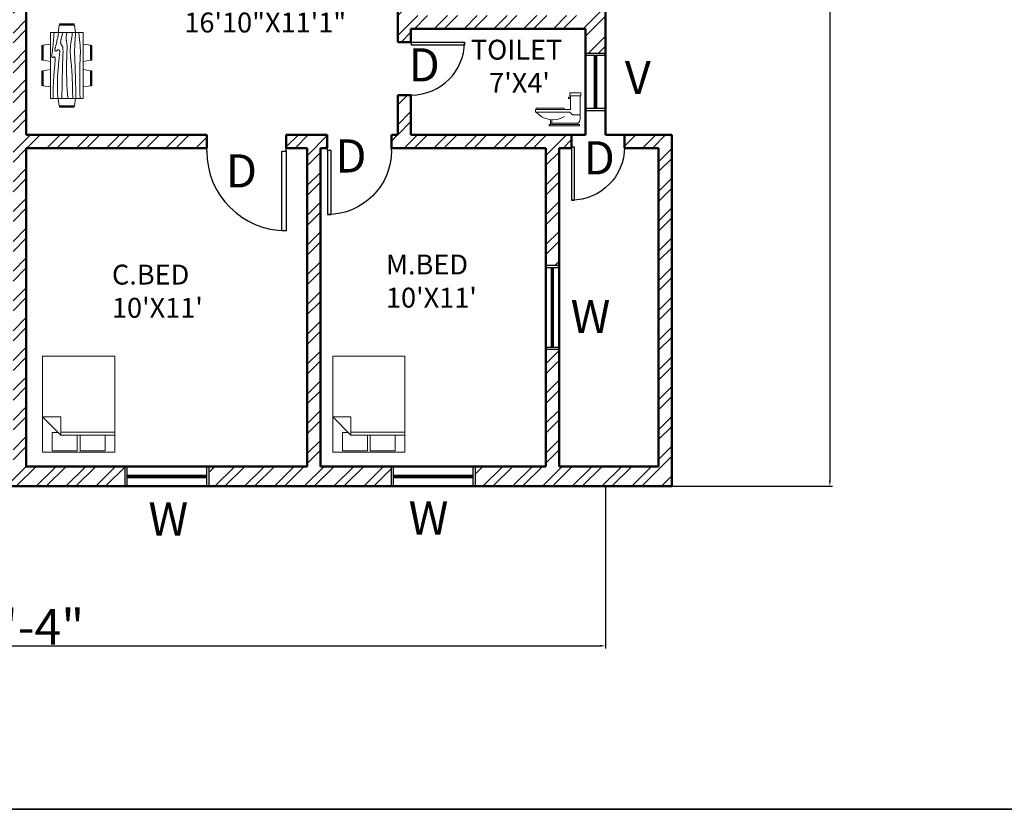
# Model space of a CAD drawing. Units: inches. Extents: x -31842 to -29388, y 18869 to 19743.
# Tile 7 of 12: x -30617 to -30172, y 18869 to 19226. Entities that reach past the tile are written whole.
import ezdxf

# ---------------------------------------------------------------- set-up
doc = ezdxf.new("R2010")
doc.units = ezdxf.units.IN
for name, color, linetype, lineweight in [('A-ANNO-DIMS', 2, 'Continuous', 18), ('A-ANNO-SYMB', 2, 'Continuous', 18), ('A-ANNO-TTLB', 7, 'Continuous', 35), ('A-AREA-IDEN', 3, 'Continuous', 18), ('A-DOOR', 3, 'Continuous', 25), ('A-FLOR-FIXT', 8, 'Continuous', 18), ('A-FURN', 8, 'Continuous', 18), ('A-GLAZ', 4, 'Continuous', 25), ('A-WALL', 7, 'Continuous', 50), ('A-WALL-PATT', 8, 'Continuous', 13)]:
    doc.layers.add(name, color=color, linetype=linetype, lineweight=lineweight)
doc.styles.get("Standard").update_dxf_attribs({"font": 'arial.ttf'})
doc.dimstyles.new('ISO-25', dxfattribs={"dimtxt": 2.5, "dimasz": 2.5, "dimexe": 1.25, "dimexo": 0.625, "dimtad": 1, "dimdec": 0, "dimlunit": 3, "dimtxsty": 'Standard', "dimcen": 2.5, "dimadec": 0, "dimazin": 0, "dimtfac": 1, "dimtdec": 0, "dimtmove": 0, "dimatfit": 3, "dimfxl": 1, "dimarcsym": 0})

# ---------------------------------------------------------------- blocks, each defined once
blk = doc.blocks.new('*U8')
for p, q in [((0, 0), (0, -100)), ((750, 0), (750, -100))]:
    blk.add_line(p, q)
blk.add_lwpolyline([(0, 0), (0, 750), (43.75, 750), (43.75, 0)], close=True)
blk.add_arc((0, 0), 750, 0, 90)
blk = doc.blocks.new('Bed - Queen')
for p, q in [((0, -80.00003), (0, 0)), ((0, 0), (59.99999, 0)), ((59.99999, 0), (59.99999, -80.00003)), ((7.99999, -1.2), (28.79998, -1.2)), ((7.99999, -14.4), (7.99999, -1.2)), ((28.79998, -1.2), (28.79998, -14.4)), ((31.19999, -1.2), (51.99999, -1.2)), ((31.19999, -14.4), (31.19999, -1.2)), ((51.99999, -1.2), (51.99999, -16.4)), ((0, -14.4), (44.8, -14.4)), ((59.99999, -29.6), (44.8, -14.4)), ((44.8, -14.4), (44.8, -29.6)), ((44.8, -16.8), (0, -16.8)), ((51.99999, -16.4), (46.79936, -16.4)), ((44.8, -29.6), (59.99999, -29.6)), ((59.99999, -80.00003), (0, -80.00003))]:
    blk.add_line(p, q)
blk = doc.blocks.new('Toilet - side')
for p, q in [((0.5, 5), (0.5, 22)), ((7.5, 22), (7.5, 12)), ((7.5, 21), (9, 21)), ((9, 20), (7.5, 20)), ((9, 21), (9, 20)), ((6, 8), (0.5, 8)), ((8, 10), (6, 8)), ((7.5, 12), (33, 12)), ((33, 10), (8, 10)), ((32.5, 13), (12, 13)), ((12, 13), (12, 12)), ((32.5, 12), (32.5, 13)), ((33, 12), (33, 10)), ((22, 2), (2, 2)), ((2, 2), (2, 1)), ((21, 4.5), (21, 2)), ((22, 2), (22, 4.54)), ((22, 1), (22, 2))]:
    blk.add_line(p, q)
for points in [[(0, 22), (0, 24), (8, 24), (8, 22)], [(1, 0), (1, 1), (23, 1), (23, 0)]]:
    blk.add_lwpolyline(points, close=True)
for centre, radius, start, end in [((20.3, 20.7), 16.23, 238.18715, 318.77023), ((3.75, 4.75), 3.26, 175.6013, 237.5288)]:
    blk.add_arc(centre, radius, start, end)
blk = doc.blocks.new('Dining Set - 36 x 72 in.')
for p, q in [((-22.2343, 26.00059), (-23.4847, 17.99762)), ((-22.2304, 26), (-5.7608, 26)), ((-22, 27.5), (-22.1562, 26.50042)), ((-5.8416, 26.5), (-22.1534, 26.5)), ((-22, 27.5), (-6, 27.5)), ((-5.8437, 26.49966), (-6, 27.5)), ((-4.5152, 17.99762), (-5.7655, 25.99926)), ((5.7657, 26.00059), (4.5153, 17.99762)), ((5.7696, 26), (22.2392, 26)), ((6, 27.5), (5.8438, 26.50042)), ((22.1584, 26.5), (5.8466, 26.5)), ((6, 27.5), (22, 27.5)), ((22.1563, 26.49966), (22, 27.5)), ((23.4848, 17.99762), (22.2345, 25.99926)), ((36, 18), (-36, 18)), ((-36, 18), (-36, -18)), ((36, -18), (36, 18)), ((-45.5, 8), (-44.5004, 8.15617)), ((-45.5, 8), (-45.5, -8)), ((-44.5, -8.15843), (-44.5, 8.15338)), ((-44.0006, 8.23428), (-35.9976, 9.48474)), ((-44, 8.23041), (-44, -8.23915)), ((44.0006, 8.23428), (35.9976, 9.48474)), ((44, 8.23041), (44, -8.23915)), ((44.5, -8.15843), (44.5, 8.15338)), ((45.5, 8), (44.5005, 8.15617)), ((45.5, 8), (45.5, -8)), ((-44.4997, -8.15631), (-45.5, -8)), ((-35.9976, -9.48476), (-43.9993, -8.2345)), ((35.9976, -9.48476), (43.9993, -8.2345)), ((44.4997, -8.15631), (45.5, -8)), ((-36, -18), (36, -18)), ((-22.2343, -26.0006), (-23.4847, -17.99762)), ((-4.5152, -17.99762), (-5.7655, -25.99928)), ((5.7657, -26.0006), (4.5153, -17.99762)), ((23.4848, -17.99762), (22.2345, -25.99928)), ((-22.2304, -26), (-5.7608, -26)), ((-22, -27.5), (-22.1562, -26.50044)), ((-5.8416, -26.5), (-22.1534, -26.5)), ((-22, -27.5), (-6, -27.5)), ((-5.8437, -26.49967), (-6, -27.5)), ((5.7696, -26), (22.2392, -26)), ((6, -27.5), (5.8438, -26.50044)), ((22.1584, -26.5), (5.8466, -26.5)), ((6, -27.5), (22, -27.5)), ((22.1563, -26.49967), (22, -27.5))]:
    blk.add_line(p, q)
for points in [[(-36, 15), (-31.1772, 14.97754), (-26.8079, 14.91406), (-22.8538, 14.81543), (-19.276, 14.6875), (-16.0362, 14.53613), (-13.0957, 14.36718), (-10.4159, 14.18652), (-7.9583, 14), (-5.6904, 13.81315), (-3.6035, 13.63021), (-1.6954, 13.45508), (0.0365, 13.29166), (1.5945, 13.14388), (2.9811, 13.01562), (4.1988, 12.9108), (5.25, 12.83333), (6.1393, 12.78613), (6.8802, 12.76823), (7.4883, 12.77767), (7.9792, 12.8125), (8.3685, 12.87077), (8.6719, 12.95052), (8.9049, 13.0498), (9.0833, 13.16666), (9.2205, 13.29899), (9.3216, 13.44401), (9.3895, 13.59879), (9.4271, 13.76041), (9.4373, 13.92594), (9.4232, 14.09245), (9.3875, 14.257), (9.3333, 14.41666), (9.2638, 14.56917), (9.1836, 14.71484), (9.0975, 14.85465), (9.0104, 14.98958), (8.9272, 15.1206), (8.8529, 15.2487), (8.7922, 15.37483), (8.75, 15.5), (8.7305, 15.62467), (8.7344, 15.74739), (8.7617, 15.86621), (8.8125, 15.97916), (8.8867, 16.08431), (8.9844, 16.17968), (9.1055, 16.26334), (9.25, 16.33333), (9.4189, 16.38802), (9.6172, 16.42708), (9.8506, 16.45052), (10.125, 16.45833), (10.4463, 16.45052), (10.8203, 16.42708), (11.2529, 16.38802), (11.75, 16.33333), (12.3184, 16.26318), (12.9694, 16.17838), (13.7151, 16.07991), (14.5677, 15.96875), (15.5395, 15.84586), (16.6426, 15.71224), (17.8893, 15.56884), (19.2917, 15.41666), (20.859, 15.25667), (22.5879, 15.08984), (24.4721, 14.91715), (26.5052, 14.73958), (28.6809, 14.5581), (30.9929, 14.3737), (33.4347, 14.18733), (36, 14)], [(-36, 10), (-28.9766, 10.14274), (-23.1725, 10.20442), (-18.4241, 10.19775), (-14.5677, 10.13541), (-11.4399, 10.03011), (-8.877, 9.89453), (-6.7154, 9.74137), (-4.7917, 9.58333), (-2.9698, 9.43082), (-1.2246, 9.28515), (0.4415, 9.14534), (2.026, 9.01041), (3.5266, 8.87939), (4.9408, 8.7513), (6.266, 8.62516), (7.5, 8.5), (8.6411, 8.37549), (9.6914, 8.2539), (10.6538, 8.13818), (11.5312, 8.03125), (12.3267, 7.93603), (13.043, 7.85547), (13.6831, 7.79248), (14.25, 7.75), (14.7471, 7.7303), (15.1797, 7.73307), (15.5537, 7.75732), (15.875, 7.80208), (16.1494, 7.86637), (16.3828, 7.94922), (16.5811, 8.04964), (16.75, 8.16666), (16.8944, 8.29915), (17.0143, 8.44531), (17.1089, 8.60319), (17.1771, 8.77083), (17.218, 8.94629), (17.2305, 9.1276), (17.2137, 9.31282), (17.1667, 9.5), (17.0895, 9.6875), (16.987, 9.875), (16.8649, 10.0625), (16.7292, 10.25), (16.5856, 10.4375), (16.4401, 10.625), (16.2985, 10.8125), (16.1667, 11), (16.05, 11.18733), (15.9518, 11.3737), (15.8752, 11.5581), (15.8229, 11.73958), (15.798, 11.91715), (15.8034, 12.08984), (15.842, 12.25667), (15.9167, 12.41666), (16.0295, 12.56836), (16.1784, 12.70833), (16.3605, 12.83268), (16.5729, 12.9375), (16.8127, 13.01888), (17.0768, 13.07291), (17.3625, 13.0957), (17.6667, 13.08333), (17.9894, 13.03312), (18.3418, 12.94726), (18.7382, 12.82918), (19.1927, 12.68229), (19.7195, 12.51001), (20.3327, 12.31575), (21.0465, 12.10294), (21.875, 11.875), (22.8357, 11.63354), (23.959, 11.37304), (25.2786, 11.08618), (26.8282, 10.76562), (28.6414, 10.40405), (30.752, 9.99414), (33.1936, 9.52856), (36, 9)], [(-36, 5.5), (-30.7157, 5.3348), (-26.069, 5.20963), (-21.9946, 5.11767), (-18.4271, 5.05208), (-15.3009, 5.00602), (-12.5508, 4.97265), (-10.1112, 4.94515), (-7.9167, 4.91666), (-5.909, 4.88167), (-4.0586, 4.83984), (-2.3429, 4.79215), (-0.7396, 4.73958), (0.7739, 4.6831), (2.22, 4.6237), (3.6213, 4.56233), (5, 4.5), (6.373, 4.43782), (7.7344, 4.3776), (9.0723, 4.32129), (10.375, 4.27083), (11.6309, 4.22819), (12.8281, 4.19531), (13.9551, 4.17415), (15, 4.16666), (15.954, 4.17448), (16.819, 4.19791), (17.6001, 4.23698), (18.3021, 4.29166), (18.9299, 4.36198), (19.4883, 4.44791), (19.9823, 4.54948), (20.4167, 4.66666), (20.7969, 4.79899), (21.1302, 4.94401), (21.4245, 5.09879), (21.6875, 5.26041), (21.9271, 5.42594), (22.1511, 5.59245), (22.3672, 5.757), (22.5834, 5.91666), (22.8065, 6.06868), (23.0404, 6.21093), (23.2879, 6.34147), (23.5521, 6.45833), (23.8358, 6.55957), (24.142, 6.64323), (24.4735, 6.70735), (24.8334, 6.75), (25.2235, 6.76969), (25.642, 6.76692), (26.0858, 6.74267), (26.5521, 6.69791), (27.0379, 6.63362), (27.5404, 6.55078), (28.0565, 6.45036), (28.5834, 6.33333), (29.1242, 6.19987), (29.7071, 6.04687), (30.3661, 5.87044), (31.1354, 5.66666), (32.0493, 5.43164), (33.142, 5.16146), (34.4475, 4.85221), (36, 4.5)], [(-36, -1), (-30.7915, -0.6591), (-26.0195, -0.38216), (-21.6519, -0.16284), (-17.6563, 0.00521), (-14.0005, 0.12833), (-10.6523, 0.21289), (-7.5796, 0.26522), (-4.75, 0.29166), (-2.134, 0.29793), (0.2878, 0.28711), (2.5317, 0.26163), (4.6146, 0.22396), (6.5529, 0.17651), (8.3633, 0.12174), (10.0623, 0.06209), (11.6667, 0), (13.1899, -0.06201), (14.6341, -0.1211), (15.9982, -0.17432), (17.2813, -0.21875), (18.4823, -0.25147), (19.6003, -0.26953), (20.6343, -0.27002), (21.5834, -0.25), (22.4481, -0.20768), (23.2357, -0.14584), (23.9549, -0.06836), (24.6146, 0.02083), (25.2235, 0.11784), (25.7904, 0.21875), (26.3241, 0.31966), (26.8334, 0.41666), (27.3265, 0.50618), (27.8099, 0.58593), (28.2894, 0.65397), (28.7709, 0.70833), (29.2601, 0.74707), (29.763, 0.76823), (30.2855, 0.76985), (30.8334, 0.75), (31.4088, 0.70784), (31.9994, 0.64713), (32.589, 0.57275), (33.1615, 0.48958), (33.7008, 0.4025), (34.1908, 0.3164), (34.6153, 0.23616), (34.9584, 0.16666), (35.2099, 0.11165), (35.3848, 0.07031), (35.504, 0.04069), (35.5886, 0.02083), (35.6594, 0.00879), (35.7377, 0.0026), (35.8442, 0.00032), (36, 0)], [(-36, -6.5), (-27.1843, -6.31267), (-20.084, -6.1263), (-14.469, -5.9419), (-10.1094, -5.76042), (-6.7752, -5.58285), (-4.2363, -5.41016), (-2.2629, -5.24333), (-0.625, -5.08334), (0.8708, -4.93099), (2.2715, -4.78646), (3.5872, -4.64974), (4.8281, -4.52084), (6.0046, -4.39974), (7.127, -4.28646), (8.2053, -4.18099), (9.25, -4.08334), (10.2705, -3.99382), (11.2734, -3.91407), (12.2647, -3.84603), (13.25, -3.79167), (14.2354, -3.75293), (15.2266, -3.73177), (16.2295, -3.73015), (17.25, -3.75), (18.2912, -3.79248), (19.3451, -3.85547), (20.4009, -3.93604), (21.4479, -4.03125), (22.4754, -4.13819), (23.4727, -4.25391), (24.4289, -4.37549), (25.3334, -4.5), (26.1785, -4.62492), (26.9694, -4.74935), (27.7145, -4.87281), (28.4219, -4.99479), (29.1, -5.11483), (29.7572, -5.23242), (30.4016, -5.34709), (31.0417, -5.45834), (31.6837, -5.56437), (32.3262, -5.65821), (32.9658, -5.73153), (33.599, -5.77604), (34.2224, -5.78345), (34.8327, -5.74545), (35.4264, -5.65373), (36, -5.5)], [(-36, -10), (-26.4022, -9.81299), (-18.4675, -9.62891), (-11.9839, -9.45069), (-6.7396, -9.28125), (-2.5226, -9.12354), (0.8789, -8.98047), (3.6769, -8.85498), (6.0833, -8.75), (8.2767, -8.66765), (10.3021, -8.60677), (12.1712, -8.56543), (13.8958, -8.54167), (15.4876, -8.53353), (16.9583, -8.53907), (18.3197, -8.55632), (19.5834, -8.58334), (20.7616, -8.61841), (21.8685, -8.66081), (22.9188, -8.71004), (23.9271, -8.76563), (24.9081, -8.82707), (25.8763, -8.89388), (26.8465, -8.96558), (27.8334, -9.04167), (28.8474, -9.12118), (29.8828, -9.20117), (30.93, -9.27824), (31.9792, -9.34896), (33.0205, -9.40991), (34.0443, -9.45768), (35.0407, -9.48885), (36, -9.5)], [(-36, -14.5), (-30.0881, -14.33513), (-25.0332, -14.21224), (-20.7312, -14.12647), (-17.0781, -14.07292), (-13.97, -14.04671), (-11.3027, -14.04297), (-8.9724, -14.05681), (-6.875, -14.08334), (-4.9224, -14.11833), (-3.0905, -14.16016), (-1.3709, -14.20785), (0.2448, -14.26042), (1.7647, -14.3169), (3.1973, -14.3763), (4.5507, -14.43767), (5.8333, -14.5), (7.0554, -14.5621), (8.235, -14.62175), (9.3922, -14.67652), (10.5469, -14.72396), (11.7192, -14.76164), (12.929, -14.78711), (14.1965, -14.79794), (15.5417, -14.79167), (16.9933, -14.76424), (18.6152, -14.70508), (20.4804, -14.60197), (22.6615, -14.44271), (25.2312, -14.21509), (28.2624, -13.9069), (31.8277, -13.50594), (36, -13)]]:
    blk.add_lwpolyline(points)
blk = doc.blocks.new('*D203')
at = {"layer": 'A-ANNO-DIMS', "color": 0, "lineweight": -2, "transparency": 16777216}
for p, q in [((-30351.77, 19614.99), (-30249.67, 19614.99)), ((-30250.92, 19612.49), (-30250.92, 19017.46)), ((-30351.77, 19014.96), (-30249.67, 19014.96))]:
    blk.add_line(p, q, dxfattribs=at)
at = {"layer": 'A-ANNO-DIMS', "color": 0, "transparency": 16777216}
for points in [[(-30251.34, 19612.49), (-30250.5, 19612.49), (-30250.92, 19614.99)], [(-30251.34, 19017.46), (-30250.5, 19017.46), (-30250.92, 19014.96)]]:
    blk.add_solid(points, dxfattribs=at)
at = {"layer": 'Defpoints', "color": 0, "transparency": 16777216}
for p in [(-30352.39, 19614.99), (-30352.39, 19014.96), (-30250.92, 19014.96)]:
    blk.add_point(p, dxfattribs=at)
at = {"layer": 'A-ANNO-DIMS', "color": 0, "transparency": 16777216, "insert": (-30259.72, 19314.97), "char_height": 2.5, "attachment_point": 5, "rotation": 90}
blk.add_mtext("{\\H6.4x;50'}", dxfattribs=at)
blk = doc.blocks.new('*D204')
at = {"layer": 'A-ANNO-DIMS', "color": 0, "lineweight": -2, "transparency": 16777216}
for p, q in [((-30884.39, 19014.34), (-30884.39, 18941.51)), ((-30352.39, 19014.34), (-30352.39, 18941.51)), ((-30881.89, 18942.76), (-30354.89, 18942.76))]:
    blk.add_line(p, q, dxfattribs=at)
at = {"layer": 'A-ANNO-DIMS', "color": 0, "transparency": 16777216}
for points in [[(-30881.89, 18943.17), (-30881.89, 18942.34), (-30884.39, 18942.76)], [(-30354.89, 18943.17), (-30354.89, 18942.34), (-30352.39, 18942.76)]]:
    blk.add_solid(points, dxfattribs=at)
at = {"layer": 'Defpoints', "color": 0, "transparency": 16777216}
for p in [(-30884.39, 19014.96), (-30352.39, 19014.96), (-30352.39, 18942.76)]:
    blk.add_point(p, dxfattribs=at)
at = {"layer": 'A-ANNO-DIMS', "color": 0, "transparency": 16777216, "insert": (-30618.39, 18951.38), "char_height": 2.5, "attachment_point": 5}
blk.add_mtext('{\\H6.4x;44\'-4"}', dxfattribs=at)
blk = doc.blocks.new('WIN-3FT')
for p, q in [((0, 36), (9, 36)), ((4, 0), (4, 36)), ((4.5, 0), (4.5, 36)), ((5, 0), (5, 36)), ((0, 0), (9, 0))]:
    blk.add_line(p, q)
blk = doc.blocks.new('WIN-3FT-B')
for p, q in [((0, 36), (6, 36)), ((2.5, 0), (2.5, 36)), ((3, 0), (3, 36)), ((3.5, 0), (3.5, 36)), ((0, 0), (6, 0))]:
    blk.add_line(p, q)
blk = doc.blocks.new('WIN-2FT')
for p, q in [((0, 24), (9, 24)), ((4, 0), (4, 24)), ((4.5, 0), (4.5, 24)), ((5, 0), (5, 24)), ((0, 0), (9, 0))]:
    blk.add_line(p, q)

msp = doc.modelspace()

# ---------------------------------------------------------------- hatches: boundary and pattern name
at = {"layer": 'A-WALL-PATT'}
h = msp.add_hatch(dxfattribs=at)
h.set_pattern_fill('ANSI32', color=256)
h.paths.add_polyline_path([(-30352.39, 19656.96), (-30487.39, 19656.96), (-30487.39, 19614.96), (-30510.39, 19614.96), (-30510.39, 19605.96), (-30487.39, 19605.96), (-30487.39, 19558.38), (-30481.39, 19558.38), (-30481.39, 19605.96), (-30469.68, 19605.96), (-30469.68, 19614.96), (-30481.39, 19614.96), (-30481.39, 19650.96), (-30361.39, 19650.96), (-30361.39, 19614.96), (-30445.68, 19614.96), (-30445.68, 19605.96), (-30361.39, 19605.96), (-30361.39, 19564.96), (-30352.39, 19564.96)])
h.paths.add_polyline_path([(-30548.39, 19614.96), (-30599.39, 19614.96), (-30599.39, 19605.96), (-30577.39, 19605.96), (-30577.39, 19457.87), (-30571.39, 19457.87), (-30571.39, 19491.96), (-30560.76, 19491.96), (-30560.76, 19497.96), (-30571.39, 19497.96), (-30571.39, 19605.96), (-30548.39, 19605.96)])
h.paths.add_polyline_path([(-30637.39, 19614.96), (-30688.39, 19614.96), (-30688.39, 19605.96), (-30665.39, 19605.96), (-30665.39, 19497.96), (-30682.48, 19497.96), (-30682.48, 19491.96), (-30665.39, 19491.96), (-30665.39, 19454.79), (-30662.43, 19454.79), (-30659.39, 19454.79), (-30659.39, 19605.96), (-30637.39, 19605.96)])
h.paths.add_polyline_path([(-30789.63, 19614.96), (-30875.39, 19614.96), (-30875.39, 19650.96), (-30755.39, 19650.96), (-30755.39, 19614.96), (-30765.63, 19614.96), (-30765.63, 19605.96), (-30755.39, 19605.96), (-30755.39, 19550.68), (-30749.39, 19550.68), (-30749.39, 19605.96), (-30726.39, 19605.96), (-30726.39, 19614.96), (-30749.39, 19614.96), (-30749.39, 19656.96), (-30884.39, 19656.96), (-30884.39, 19564.96), (-30875.39, 19564.96), (-30875.39, 19605.96), (-30789.63, 19605.96)])
h.paths.add_polyline_path([(-30749.39, 19491.96), (-30736.92, 19491.96), (-30736.92, 19494.96), (-30682.48, 19494.96), (-30682.48, 19497.96), (-30665.39, 19497.96), (-30665.39, 19605.96), (-30688.39, 19605.96), (-30749.39, 19605.96), (-30749.39, 19550.68), (-30755.39, 19550.68), (-30757.34, 19550.71, 0.39722), (-30793.34, 19516.76), (-30757.34, 19516.76), (-30757.34, 19514.65), (-30793.4, 19514.65), (-30793.4, 19516.76), (-30793.34, 19516.76, -0.39722), (-30757.34, 19550.71), (-30755.39, 19550.71), (-30755.39, 19605.96), (-30765.63, 19605.96), (-30765.63, 19613.66), (-30767.03, 19613.66), (-30767.03, 19637.62, 0.397344), (-30789.63, 19613.65), (-30789.63, 19605.96), (-30875.39, 19605.96), (-30875.39, 19564.96), (-30875.39, 19485.96), (-30873.79, 19485.96), (-30873.79, 19479.96), (-30873.79, 19479.35, 0.39722), (-30851.19, 19455.39), (-30851.19, 19479.35), (-30849.79, 19479.35), (-30849.79, 19455.34), (-30851.19, 19455.34), (-30851.19, 19455.39, -0.39722), (-30873.79, 19479.35), (-30873.79, 19479.96), (-30875.39, 19479.96), (-30875.39, 19431.96), (-30848.39, 19431.96), (-30848.39, 19468.96), (-30842.39, 19468.96), (-30842.39, 19479.96), (-30755.39, 19479.96), (-30755.39, 19470.97), (-30749.39, 19470.97)])
h.paths.add_polyline_path([(-30738.39, 19585.51), (-30738.39, 19586.08), (-30736.12, 19586.08), (-30736.12, 19586.65), (-30739.53, 19586.65), (-30739.53, 19600.27), (-30722.5, 19600.27), (-30722.5, 19586.65), (-30725.91, 19586.65), (-30725.91, 19586.08), (-30723.64, 19586.08), (-30723.64, 19585.51)], flags=16)
h.paths.add_polyline_path([(-30737.83, 19590.05, -1), (-30734.42, 19590.05, -1)], flags=16)
h.paths.add_polyline_path([(-30737.26, 19590.05, -1), (-30734.99, 19590.05, -1)], flags=0)
h.paths.add_polyline_path([(-30732.72, 19588.35), (-30732.72, 19597.43), (-30729.31, 19597.43), (-30729.31, 19588.35)], flags=16)
h.paths.add_polyline_path([(-30736.69, 19590.05, -1), (-30735.56, 19590.05, -1)], flags=0)
h.paths.add_polyline_path([(-30732.15, 19588.92), (-30732.15, 19596.86), (-30729.88, 19596.86), (-30729.88, 19588.92)], flags=0)
h.paths.add_polyline_path([(-30728.18, 19590.05, -1), (-30723.64, 19590.05, -1)], flags=0)
h.paths.add_polyline_path([(-30727.61, 19590.05, -1), (-30724.2, 19590.05, -1)], flags=0)
h.paths.add_polyline_path([(-30727.04, 19590.05, -1), (-30724.77, 19590.05, -1)], flags=0)
h.paths.add_polyline_path([(-30726.47, 19590.05, -1), (-30725.34, 19590.05, -1)], flags=0)
h.paths.add_polyline_path([(-30738.39, 19595.16, -1), (-30733.85, 19595.16, -1)], flags=16)
h.paths.add_polyline_path([(-30737.83, 19595.16, -1), (-30734.42, 19595.16, -1)], flags=0)
h.paths.add_polyline_path([(-30737.26, 19595.16, -1), (-30734.99, 19595.16, -1)], flags=0)
h.paths.add_polyline_path([(-30736.69, 19595.16, -1), (-30735.56, 19595.16, -1)], flags=0)
h.paths.add_polyline_path([(-30727.61, 19595.16, -1), (-30724.2, 19595.16, -1)], flags=0)
h.paths.add_polyline_path([(-30727.04, 19595.16, -1), (-30724.77, 19595.16, -1)], flags=0)
h.paths.add_polyline_path([(-30707.55, 19587.34, -0.414214), (-30708.36, 19588.14), (-30708.36, 19597.29, -0.414214), (-30707.55, 19598.09), (-30693.03, 19598.09, -0.414214), (-30692.23, 19597.29), (-30692.23, 19588.14, -0.414214), (-30693.03, 19587.34)], flags=16)
h.paths.add_polyline_path([(-30726.47, 19595.16, -1), (-30725.34, 19595.16, -1)], flags=0)
h.paths.add_polyline_path([(-30827.74, 19570.11), (-30871.22, 19570.11), (-30871.22, 19602.72), (-30827.74, 19602.72)], flags=16)
h.paths.add_polyline_path([(-30707.01, 19588.14, -0.414214), (-30707.55, 19588.68), (-30707.55, 19594.6, -0.414214), (-30707.01, 19595.13), (-30693.57, 19595.13, -0.414214), (-30693.03, 19594.6), (-30693.03, 19588.68, -0.414214), (-30693.57, 19588.14)], flags=0)
h.paths.add_polyline_path([(-30700.02, 19591.64, -1), (-30700.56, 19591.64, -1)], flags=0)
h.paths.add_polyline_path([(-30863.39, 19594.46), (-30863.39, 19574.46), (-30870.57, 19574.46), (-30870.57, 19585.76), (-30863.39, 19585.76), (-30863.39, 19587.07), (-30870.57, 19587.07), (-30870.57, 19598.37), (-30862.31, 19598.37), (-30862.31, 19595.55), (-30855.13, 19602.72), (-30855.13, 19594.46)], flags=0)
h.paths.add_polyline_path([(-30755.39, 19514.65), (-30757.34, 19514.65), (-30793.4, 19514.65), (-30793.4, 19516.76), (-30793.34, 19516.76, -0.39722), (-30757.34, 19550.71), (-30755.39, 19550.71), (-30755.39, 19605.96), (-30765.63, 19605.96), (-30765.63, 19613.66), (-30767.03, 19613.66), (-30767.03, 19637.62, 0.397344), (-30789.63, 19613.65), (-30789.63, 19605.96), (-30875.39, 19605.96), (-30875.39, 19564.96), (-30875.39, 19485.96), (-30873.79, 19485.96), (-30873.79, 19479.96), (-30873.79, 19479.35, 0.39722), (-30851.19, 19455.39), (-30851.19, 19479.35), (-30849.79, 19479.35), (-30849.79, 19479.96), (-30849.79, 19479.96), (-30849.79, 19485.96), (-30755.39, 19485.96)], flags=16)
h.paths.add_polyline_path([(-30665.39, 19605.96), (-30688.39, 19605.96), (-30749.39, 19605.96), (-30749.39, 19550.68), (-30755.39, 19550.68), (-30757.34, 19550.71, 0.39722), (-30793.34, 19516.76), (-30757.34, 19516.76), (-30757.34, 19514.65), (-30755.39, 19514.65), (-30755.39, 19514.68), (-30749.39, 19514.68), (-30749.39, 19497.96), (-30736.92, 19497.96), (-30736.92, 19494.96), (-30682.48, 19494.96), (-30682.48, 19497.96), (-30665.39, 19497.96)], flags=17)
h.paths.add_polyline_path([(-30749.39, 19446.97), (-30755.39, 19446.97), (-30755.39, 19431.96), (-30842.39, 19431.96), (-30842.39, 19442.96), (-30848.39, 19442.96), (-30848.39, 19431.96), (-30875.39, 19431.96), (-30875.39, 19479.96), (-30873.79, 19479.96), (-30873.79, 19482.55), (-30873.79, 19485.96), (-30875.39, 19485.96), (-30875.39, 19526.96), (-30884.39, 19526.96), (-30884.39, 19384.96), (-30875.39, 19384.96), (-30875.39, 19425.96), (-30755.39, 19425.96), (-30755.39, 19414.67), (-30751.3, 19414.67), (-30749.39, 19414.62)])
h.paths.add_polyline_path([(-30848.39, 19468.96), (-30848.39, 19479.96), (-30849.79, 19479.96), (-30849.79, 19479.35), (-30849.79, 19455.34), (-30851.19, 19455.34), (-30851.19, 19455.39, -0.39722), (-30873.79, 19479.35), (-30873.79, 19479.96), (-30875.39, 19479.96), (-30875.39, 19431.96), (-30848.39, 19431.96), (-30848.39, 19442.96)], flags=17)
h.paths.add_polyline_path([(-30659.39, 19407.96), (-30657.22, 19407.96), (-30657.22, 19413.96), (-30659.39, 19413.96), (-30659.39, 19418.79), (-30665.39, 19418.79), (-30665.39, 19305.96), (-30749.39, 19305.96), (-30749.39, 19378.62), (-30755.39, 19378.62), (-30755.39, 19305.96), (-30875.39, 19305.96), (-30875.39, 19346.96), (-30884.39, 19346.96), (-30884.39, 19282.96), (-30875.39, 19282.96), (-30875.39, 19299.96), (-30796.39, 19299.96), (-30796.39, 19286.68), (-30790.39, 19286.68), (-30790.39, 19299.96), (-30659.39, 19299.96)])
h.paths.add_polyline_path([(-30352.39, 19346.96), (-30361.39, 19346.96), (-30361.39, 19305.96), (-30481.39, 19305.96), (-30481.39, 19380.1), (-30487.39, 19380.1), (-30487.39, 19305.96), (-30571.39, 19305.96), (-30571.39, 19421.87), (-30577.39, 19421.87), (-30577.39, 19413.96), (-30579.53, 19413.96), (-30579.53, 19407.96), (-30577.39, 19407.96), (-30577.39, 19299.96), (-30446.39, 19299.96), (-30446.39, 19291.76), (-30440.39, 19291.76), (-30440.39, 19299.96), (-30361.39, 19299.96), (-30361.39, 19282.96), (-30352.39, 19282.96)])
h.paths.add_polyline_path([(-30481.39, 19449.62), (-30484.39, 19449.62), (-30487.39, 19449.62), (-30487.39, 19416.1), (-30481.39, 19416.1), (-30481.39, 19425.96), (-30361.39, 19425.96), (-30361.39, 19384.96), (-30352.39, 19384.96), (-30352.39, 19526.96), (-30361.39, 19526.96), (-30361.39, 19485.96), (-30363.32, 19485.96), (-30363.32, 19479.96), (-30361.39, 19479.96), (-30361.39, 19431.96), (-30388.39, 19431.96), (-30388.39, 19442.96), (-30394.39, 19442.96), (-30394.39, 19431.96), (-30481.39, 19431.96)])
h.paths.add_polyline_path([(-30387.32, 19482.76), (-30387.32, 19485.96), (-30481.39, 19485.96), (-30481.39, 19522.38), (-30487.39, 19522.38), (-30487.39, 19497.96), (-30500.08, 19497.96), (-30500.08, 19491.96), (-30487.39, 19491.96), (-30487.39, 19473.62), (-30481.39, 19473.62), (-30481.39, 19479.96), (-30394.39, 19479.96), (-30394.39, 19468.96), (-30388.39, 19468.96), (-30388.39, 19479.96), (-30387.32, 19479.96)])
h.paths.add_polyline_path([(-30626.04, 19413.96), (-30610.58, 19413.96), (-30610.58, 19407.24), (-30608.81, 19407.24), (-30608.81, 19376.14), (-30610.63, 19376.14), (-30610.63, 19407.96), (-30614.39, 19407.96), (-30614.39, 19173.96), (-30532.79, 19173.96), (-30532.79, 19167.96), (-30532.79, 19166.59), (-30532.79, 19167.96), (-30614.39, 19167.96), (-30614.39, 19023.96), (-30568.89, 19023.96), (-30568.89, 19014.96), (-30666.89, 19014.96), (-30666.89, 19018.96), (-30702.89, 19018.96), (-30702.89, 19019.96), (-30666.89, 19019.96), (-30666.89, 19023.96), (-30620.39, 19023.96), (-30620.39, 19167.96), (-30707.45, 19167.96), (-30707.45, 19166.65, -0.39722), (-30741.49, 19130.57), (-30741.49, 19130.51), (-30743.6, 19130.51), (-30743.6, 19166.65), (-30741.49, 19166.65), (-30741.49, 19130.57, 0.407721), (-30707.48, 19167.96), (-30707.53, 19167.96), (-30707.53, 19173.96), (-30620.39, 19173.96), (-30620.39, 19407.96), (-30626.04, 19407.96), (-30626.04, 19406.62), (-30626.04, 19375.45), (-30627.86, 19375.45), (-30627.86, 19406.62), (-30626.04, 19406.62), (-30626.04, 19407.96), (-30626.04, 19407.96)])
h.paths.add_polyline_path([(-30481.39, 19167.96), (-30478.24, 19167.96), (-30478.24, 19173.96), (-30487.39, 19173.96), (-30496.79, 19173.96), (-30496.79, 19167.96), (-30487.39, 19167.96), (-30487.39, 19023.96), (-30531.89, 19023.96), (-30531.89, 19014.96), (-30449.39, 19014.96), (-30449.39, 19023.96), (-30481.39, 19023.96)])
h.paths.add_polyline_path([(-30322.39, 19173.96), (-30343.77, 19173.96), (-30343.77, 19167.96), (-30328.39, 19167.96), (-30328.39, 19023.96), (-30373.39, 19023.96), (-30373.39, 19076.96), (-30379.39, 19076.96), (-30379.39, 19023.96), (-30411.39, 19023.96), (-30411.39, 19014.96), (-30322.39, 19014.96)])
h.paths.add_polyline_path([(-30367.77, 19173.96), (-30440.39, 19173.96), (-30440.39, 19191.96), (-30446.39, 19191.96), (-30446.39, 19173.96), (-30449.24, 19173.96), (-30449.24, 19167.96), (-30379.39, 19167.96), (-30379.39, 19114.96), (-30373.39, 19114.96), (-30373.39, 19167.96), (-30367.77, 19167.96)])
h.paths.add_polyline_path([(-30857.39, 19167.96), (-30814.74, 19167.96), (-30787.91, 19167.96), (-30787.91, 19173.96), (-30790.39, 19173.96), (-30790.39, 19191.02), (-30796.39, 19191.02), (-30796.39, 19173.96), (-30814.74, 19173.96), (-30871.78, 19173.96), (-30871.78, 19167.96), (-30863.39, 19167.96), (-30863.39, 19114.96), (-30857.39, 19114.96)])
h.paths.add_polyline_path([(-30857.39, 19076.96), (-30863.39, 19076.96), (-30863.39, 19023.96), (-30908.39, 19023.96), (-30908.39, 19167.96), (-30895.78, 19167.96), (-30895.78, 19173.96), (-30914.39, 19173.96), (-30914.39, 19014.96), (-30825.39, 19014.96), (-30825.39, 19023.96), (-30857.39, 19023.96)])
h.paths.add_polyline_path([(-30758.91, 19173.96), (-30743.53, 19173.96), (-30743.53, 19167.96), (-30743.6, 19166.65), (-30741.49, 19166.65), (-30741.49, 19130.51), (-30743.6, 19130.51), (-30743.6, 19166.65), (-30743.6, 19167.96), (-30749.39, 19167.96), (-30749.39, 19023.96), (-30702.89, 19023.96), (-30702.89, 19019.46), (-30666.89, 19019.46), (-30666.89, 19018.96), (-30702.89, 19018.96), (-30702.89, 19014.96), (-30788.39, 19014.96), (-30788.39, 19018.96), (-30824.39, 19018.96), (-30824.39, 19019.96), (-30788.39, 19019.96), (-30788.39, 19023.96), (-30755.39, 19023.96), (-30755.39, 19167.96), (-30758.91, 19167.96), (-30758.91, 19166.97), (-30758.91, 19137.97), (-30760.6, 19137.97), (-30760.6, 19166.97), (-30758.91, 19166.97), (-30758.91, 19167.96), (-30758.91, 19167.96)])
h.paths.add_polyline_path([(-30790.39, 19237.4), (-30796.39, 19237.4), (-30796.39, 19227.96), (-30875.39, 19227.96), (-30875.39, 19244.96), (-30884.39, 19244.96), (-30884.39, 19210.96), (-30875.39, 19210.96), (-30875.39, 19221.96), (-30796.39, 19221.96), (-30796.39, 19215.02), (-30793.87, 19215.02), (-30790.39, 19215.02)])
h.paths.add_polyline_path([(-30352.39, 19244.96), (-30361.39, 19244.96), (-30361.39, 19227.96), (-30440.39, 19227.96), (-30440.39, 19236.96), (-30446.39, 19236.96), (-30446.39, 19215.96), (-30440.39, 19215.96), (-30440.39, 19221.96), (-30361.39, 19221.96), (-30361.39, 19210.96), (-30352.39, 19210.96)])
h.paths.add_polyline_path([(-30788.99, 19602.36), (-30766.36, 19602.36), (-30766.36, 19633.27), (-30788.99, 19633.27)], flags=24)
h.paths.add_polyline_path([(-30871.43, 19460.05), (-30848.8, 19460.05), (-30848.8, 19490.96), (-30871.43, 19490.96)], flags=24)
h.paths.add_polyline_path([(-30778.82, 19519.23), (-30756.18, 19519.23), (-30756.18, 19550.14), (-30778.82, 19550.14)], flags=24)
h.paths.add_polyline_path([(-30741.54, 19533.68), (-30681.86, 19533.68), (-30681.86, 19567.23), (-30741.54, 19567.23)], flags=24)
h.paths.add_polyline_path([(-30866.65, 19526.15), (-30802.54, 19526.15), (-30802.54, 19559.73), (-30866.65, 19559.73)], flags=8)

# ---------------------------------------------------------------- linework, layer by layer
at = {"layer": 'A-ANNO-TTLB'}
msp.add_lwpolyline([(-31842.18, 19743.36), (-29387.67, 19743.36), (-29387.67, 18868.82), (-31842.18, 18868.82)], close=True, dxfattribs=at)
at = {"layer": 'A-GLAZ'}
for p, q in [((-30361.39, 19210.96), (-30352.39, 19210.96)), ((-30361.39, 19184.96), (-30352.39, 19184.96)), ((-30379.39, 19114.96), (-30373.39, 19114.96)), ((-30379.39, 19076.96), (-30373.39, 19076.96)), ((-30569.89, 19023.96), (-30569.89, 19014.96)), ((-30531.89, 19023.96), (-30531.89, 19014.96)), ((-30449.39, 19023.96), (-30449.39, 19014.96)), ((-30411.39, 19023.96), (-30411.39, 19014.96))]:
    msp.add_line(p, q, dxfattribs=at)
at = {"layer": 'A-WALL'}
for p, q in [((-30352.39, 19656.96), (-30352.39, 19173.96)), ((-30614.39, 19173.96), (-30614.39, 19407.96)), ((-30446.39, 19236.96), (-30446.39, 19215.96)), ((-30440.39, 19221.96), (-30361.39, 19221.96)), ((-30440.39, 19221.96), (-30440.39, 19215.96)), ((-30361.39, 19221.96), (-30361.39, 19173.96)), ((-30446.39, 19215.96), (-30440.39, 19215.96)), ((-30446.39, 19191.96), (-30440.39, 19191.96)), ((-30446.39, 19191.96), (-30446.39, 19173.96)), ((-30440.39, 19191.96), (-30440.39, 19173.96)), ((-30614.39, 19173.96), (-30532.79, 19173.96)), ((-30532.79, 19167.96), (-30532.79, 19173.96)), ((-30496.79, 19167.96), (-30496.79, 19173.96)), ((-30496.79, 19173.96), (-30478.24, 19173.96)), ((-30487.39, 19173.96), (-30478.24, 19173.96)), ((-30478.24, 19167.96), (-30478.24, 19173.96)), ((-30449.24, 19167.96), (-30449.24, 19173.96)), ((-30449.24, 19173.96), (-30446.39, 19173.96)), ((-30449.24, 19173.96), (-30446.39, 19173.96)), ((-30440.39, 19173.96), (-30361.39, 19173.96)), ((-30367.77, 19173.96), (-30367.77, 19167.96)), ((-30352.39, 19173.96), (-30322.39, 19173.96)), ((-30343.77, 19173.96), (-30343.77, 19167.96)), ((-30322.39, 19173.96), (-30322.39, 19014.96)), ((-30614.39, 19023.96), (-30614.39, 19167.96)), ((-30614.39, 19167.96), (-30532.79, 19167.96)), ((-30496.79, 19167.96), (-30487.39, 19167.96)), ((-30487.39, 19167.96), (-30487.39, 19023.96)), ((-30481.39, 19167.96), (-30478.24, 19167.96)), ((-30481.39, 19167.96), (-30481.39, 19023.96)), ((-30481.39, 19167.96), (-30478.24, 19167.96)), ((-30449.24, 19167.96), (-30446.39, 19167.96)), ((-30449.24, 19167.96), (-30379.39, 19167.96)), ((-30379.39, 19167.96), (-30379.39, 19023.96)), ((-30373.39, 19167.96), (-30373.39, 19023.96)), ((-30373.39, 19167.96), (-30367.77, 19167.96)), ((-30343.77, 19167.96), (-30328.39, 19167.96)), ((-30328.39, 19167.96), (-30328.39, 19023.96)), ((-30487.39, 19023.96), (-30614.39, 19023.96)), ((-30379.39, 19023.96), (-30481.39, 19023.96)), ((-30328.39, 19023.96), (-30373.39, 19023.96)), ((-30322.39, 19014.96), (-30914.39, 19014.96))]:
    msp.add_line(p, q, dxfattribs=at)

# ---------------------------------------------------------------- block references
at = {"layer": 'A-DOOR'}
for p, xscale, yscale, zscale, rotation in [((-30440.19, 19215.96), 0.0320000008125469, 0.0320000008125469, 0.0320000008125469, 270), ((-30496.79, 19166.59), 0.0480024923977823, 0.0480024923977823, 0.0480024923977823, 180), ((-30478.2, 19166.85), -0.0386196857709081, 0.0386196857709081, 0.0386196857709081, 180), ((-30367.82, 19168.44), -0.03199974142424, 0.03199974142424, 0.03199974142424, 180)]:
    msp.add_blockref('*U8', p, dxfattribs=dict(at, xscale=xscale, yscale=yscale, zscale=zscale, rotation=rotation))
at = {"layer": 'A-FLOR-FIXT', "xscale": -0.6210234921067381, "yscale": 0.6210234921067381, "zscale": 0.6210234921067381}
msp.add_blockref('Toilet - side', (-30363.61, 19177.99), dxfattribs=at)
at = {"layer": 'A-FURN'}
for name, p, xscale, yscale, zscale, rotation in [('Dining Set - 36 x 72 in.', (-30596.07, 19205.33), 0.4136315660595786, 0.4136315660595786, 0.4136315660595786, 90), ('Bed - Queen', (-30574.41, 19030.33), 0.5435212084103092, 0.5435212084103092, 0.5435212084103092, 180), ('Bed - Queen', (-30443.18, 19030.33), 0.5435212084103092, 0.5435212084103092, 0.5435212084103092, 180)]:
    msp.add_blockref(name, p, dxfattribs=dict(at, xscale=xscale, yscale=yscale, zscale=zscale, rotation=rotation))
at = {"layer": 'A-GLAZ'}
for name, p in [('WIN-2FT', (-30361.39, 19185.96)), ('WIN-3FT-B', (-30379.39, 19077.96))]:
    msp.add_blockref(name, p, dxfattribs=at)
at = {"layer": 'A-GLAZ', "rotation": 269.9999999999782}
for p in [(-30568.89, 19023.96), (-30448.39, 19023.96)]:
    msp.add_blockref('WIN-3FT', p, dxfattribs=at)

# ---------------------------------------------------------------- texts
at = {"layer": 'A-ANNO-SYMB', "char_height": 15, "attachment_point": 1}
for s, insert in [('{D}', (-30441.47, 19213.12)), ('{V}', (-30343.68, 19207.43)), ('{D}', (-30474.59, 19171.92)), ('{D}', (-30362.29, 19171.06)), ('{D}', (-30524.12, 19165.15)), ('{W}', (-30368.18, 19099.28)), ('{W}', (-30559.16, 19007.64)), ('{W}', (-30441.45, 19008.08))]:
    msp.add_mtext_dynamic_manual_height_columns(s, width=971.0743, gutter_width=12.5, heights=[0], dxfattribs=dict(at, insert=insert))
at = {"layer": 'A-AREA-IDEN', "char_height": 9, "attachment_point": 1}
for s, insert in [('{LIVING/DINING\\P  16\'10"X11\'1"}', (-30548.42, 19244.27)), ("{    TOILET\\P       7'X4'}", (-30424.3, 19216.98)), ("{   M.BED\\P   10'X11'}", (-30459.97, 19119.81)), ("{   C.BED\\P   10'X11'}", (-30583.91, 19115.22))]:
    msp.add_mtext_dynamic_manual_height_columns(s, width=1016.678, gutter_width=12.5, heights=[0], dxfattribs=dict(at, insert=insert))

# ---------------------------------------------------------------- dimensions: what is measured, and where the dimension line sits
at = {"layer": 'A-ANNO-DIMS'}
dim = msp.add_linear_dim(base=(-30250.92, 19014.96), p1=(-30352.39, 19614.99), p2=(-30352.39, 19014.96), angle=90, text='{\\H6.4x;<>}', dimstyle='ISO-25', override={"dimclrd": 0, "dimclre": 0, "dimclrt": 0}, dxfattribs=at)
dim.commit()
dim.dimension.update_dxf_attribs({"geometry": '*D203', "text_midpoint": (-30259.72, 19314.97)})
dim = msp.add_linear_dim(base=(-30352.39, 18942.76), p1=(-30884.39, 19014.96), p2=(-30352.39, 19014.96), text='{\\H6.4x;<>}', dimstyle='ISO-25', override={"dimclrd": 0, "dimclre": 0, "dimclrt": 0}, dxfattribs=at)
dim.commit()
dim.dimension.update_dxf_attribs({"geometry": '*D204', "text_midpoint": (-30618.39, 18951.38)})

doc.saveas('drawing.dxf')
